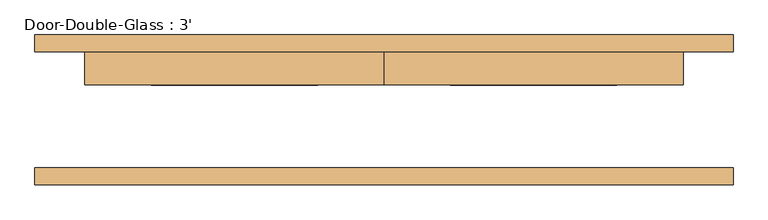
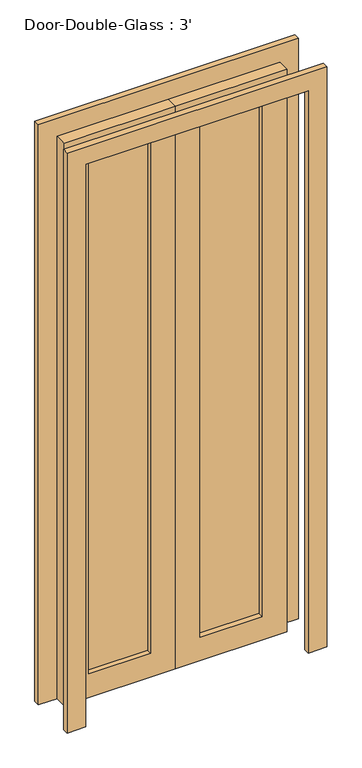
"""IFC4 building model written with IfcOpenShell, lengths in millimetres: door geometry, Door-Double-Glass : 3'."""

from ifc_helpers import new_model, si_unit, frame, origin, place, context, project, spatial, polyline, outline, extrude, source, transform, mapped, element, save


def door_double_glass_3_725c6459(model_context):
    return source(origin(), model_context, "Body", "SweptSolid", [
        extrude(outline(polyline([(2438.4, 457.2), (2438.4, 0.0), (0.0, 0.0), (0.0, 457.2), (2438.4, 457.2)]), holes=[polyline([(2336.8, 355.6), (101.6, 355.6), (101.6, 101.6), (2336.8, 101.6), (2336.8, 355.6)])]), frame((0.0, 40.48125, 0.0), z_axis=(0.0, 1.0, 0.0), x_axis=(0.0, 0.0, 1.0)), (0.0, 0.0, 1.0), 50.8),
        extrude(outline(polyline([(2438.4, -457.2), (0.0, -457.2), (0.0, 0.0), (2438.4, 0.0), (2438.4, -457.2)]), holes=[polyline([(2336.8, -355.6), (2336.8, -101.6), (101.6, -101.6), (101.6, -355.6), (2336.8, -355.6)])]), frame((0.0, 40.48125, 0.0), z_axis=(0.0, 1.0, 0.0), x_axis=(0.0, 0.0, 1.0)), (0.0, 0.0, 1.0), 50.8),
        extrude(outline(polyline([(-355.6, 69.05625), (-101.6, 69.05625), (-101.6, 62.70625), (-355.6, 62.70625), (-355.6, 69.05625)])), frame((0.0, 0.0, 101.6), z_axis=(0.0, 0.0, 1.0), x_axis=(1.0, 0.0, 0.0)), (0.0, 0.0, 1.0), 2235.2),
        extrude(outline(polyline([(101.6, 69.05625), (355.6, 69.05625), (355.6, 62.70625), (101.6, 62.70625), (101.6, 69.05625)])), frame((0.0, 0.0, 101.6), z_axis=(0.0, 0.0, 1.0), x_axis=(1.0, 0.0, 0.0)), (0.0, 0.0, 1.0), 2235.2),
        extrude(outline(polyline([(0.0, 533.4), (2514.6, 533.4), (2514.6, -533.4), (0.0, -533.4), (0.0, -457.2), (2438.4, -457.2), (2438.4, 457.2), (0.0, 457.2), (0.0, 533.4)])), frame((0.0, -111.91875, 0.0), z_axis=(0.0, 1.0, 0.0), x_axis=(0.0, 0.0, 1.0)), (0.0, 0.0, 1.0), 25.4),
        extrude(outline(polyline([(0.0, 533.4), (2514.6, 533.4), (2514.6, -533.4), (0.0, -533.4), (0.0, -457.2), (2438.4, -457.2), (2438.4, 457.2), (0.0, 457.2), (0.0, 533.4)])), frame((0.0, 91.28125, 0.0), z_axis=(0.0, 1.0, 0.0), x_axis=(0.0, 0.0, 1.0)), (0.0, 0.0, 1.0), 25.4),
    ])


if __name__ == "__main__":
    model = new_model("IFC4")
    model_context = context("Model", 3, world=origin())
    ifc_project = project(units=[si_unit("LENGTHUNIT", "METRE", prefix="MILLI")], contexts=[model_context])
    site = spatial("IfcSite", under=ifc_project)
    building = spatial("IfcBuilding", under=site)
    placement = place(None, origin())
    door_double_glass_3_shape = door_double_glass_3_725c6459(model_context)
    element("IfcDoor", 1, ObjectType="Door-Double-Glass : 3'", at=placement, inside=building, context=model_context, shape_type="MappedRepresentation", body=[
        mapped(door_double_glass_3_shape, transform((0.0, 0.0, 0.0), x_axis=(1.0, 0.0, 0.0), y_axis=(0.0, 1.0, 0.0), z_axis=(0.0, 0.0, 1.0))),
    ])
    save(model, "model.ifc")

# Revit data of these elements
# Type "Door-Double-Glass : 3'"
#   Type Mark = "14"
#   Construction Type Id = "opn-d45"
#   Assembly Code = "C1020"
#   Analytic Construction = "Wood frame, double glass door "
#   W = 1' - 6"
#   Thickness = 0' - 2"
#   Thermal Resistance (R) = 1.8150 (h·ft²·°F)/BTU
#   Swing Angle [instance default] = 90.00°
#   Heat Transfer Coefficient (U) = 0.5510 BTU/(h·ft²·°F)
#   Height = 8' - 0"
#   Bottom Rail = 0' - 4"
#   Top Rail = 0' - 4"
#   Stiles = 0' - 4"
#   Trim Projection = 0' - 1"
#   Trim Width = 0' - 3"
#   Width = 3' - 0"
#   Define Thermal Properties by = 1
#   Glazing = Glass
#   Panel Material = Wood - Birch - Solid Stained Light Low Gloss
#   Trim Material = Paint - Sienna
#   Visual Light Transmittance = 0
#   Solar Heat Gain Coefficient = 0
#   Function = (empty or 0)
#   Wall Closure = (empty or 0)
# Element 1 (IfcDoor, "Door-Double-Glass : 3'")
#   Materials on its faces: "Wood - Birch - Solid Stained Light Low Gloss", "Paint - Sienna", "Glass"
# Materials
#   "Glass": class "Glass", colour RGB 0 128 192, transparency 0.75, Description = "Soda Lime Glass", Cost = 0
#   "Wood - Birch - Solid Stained Light Low Gloss": class "Wood", colour RGB 210 159 95, transparency 0, Cost = 0
#   "Paint - Sienna": colour RGB 118 70 51, transparency 0, Cost = 0
